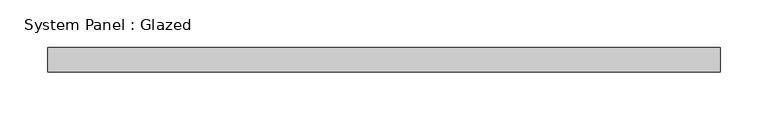
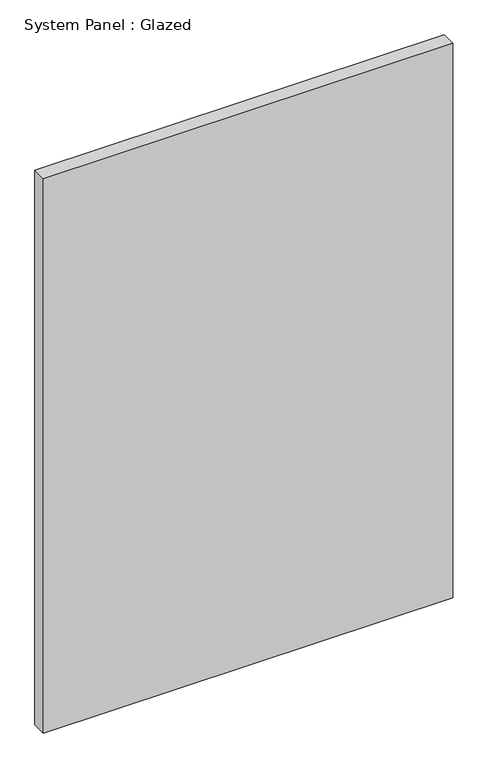
"""IFC4 building model written with IfcOpenShell, lengths in millimetres: plate geometry, System Panel : Glazed."""

from ifc_helpers import new_model, si_unit, origin, origin_with_axes, place, context, project, spatial, polyline, outline, extrude, source, transform, mapped, element, save


def system_panel_glazed_68e8fd94(model_context):
    return source(origin(), model_context, "Body", "SweptSolid", [
        extrude(outline(polyline([(350.3083333, 19.05), (-350.3083333, 19.05), (-350.3083333, 44.45), (350.3083333, 44.45), (350.3083333, 19.05)])), origin_with_axes(), (0.0, 0.0, 1.0), 1003.3),
    ])


if __name__ == "__main__":
    model = new_model("IFC4")
    model_context = context("Model", 3, world=origin())
    ifc_project = project(units=[si_unit("LENGTHUNIT", "METRE", prefix="MILLI")], contexts=[model_context])
    site = spatial("IfcSite", under=ifc_project)
    building = spatial("IfcBuilding", under=site)
    placement = place(None, origin())
    system_panel_glazed_shape = system_panel_glazed_68e8fd94(model_context)
    element("IfcPlate", 1, ObjectType="System Panel : Glazed", at=placement, inside=building, context=model_context, shape_type="MappedRepresentation", body=[
        mapped(system_panel_glazed_shape, transform((0.0, 0.0, 0.0), x_axis=(1.0, 0.0, 0.0), y_axis=(0.0, 1.0, 0.0), z_axis=(0.0, 0.0, 1.0))),
    ])
    save(model, "model.ifc")

# Revit data of these elements
# Type "System Panel : Glazed"
#   Construction Type Id = "GSP4R"
#   Analytic Construction = "1/8 in Pilkington single glazing"
#   Visual Light Transmittance = 0.9
#   Solar Heat Gain Coefficient = 0.86
#   Heat Transfer Coefficient (U) = 1.18115 BTU/(h·ft²·°F)
# Element 1 (IfcPlate, "System Panel : Glazed")
#   Materials on its faces: "Glass"
# Materials
#   "Glass": class "Glass", colour RGB 0 128 192, transparency 0.75, Description = "Soda Lime Glass", Cost = 0
